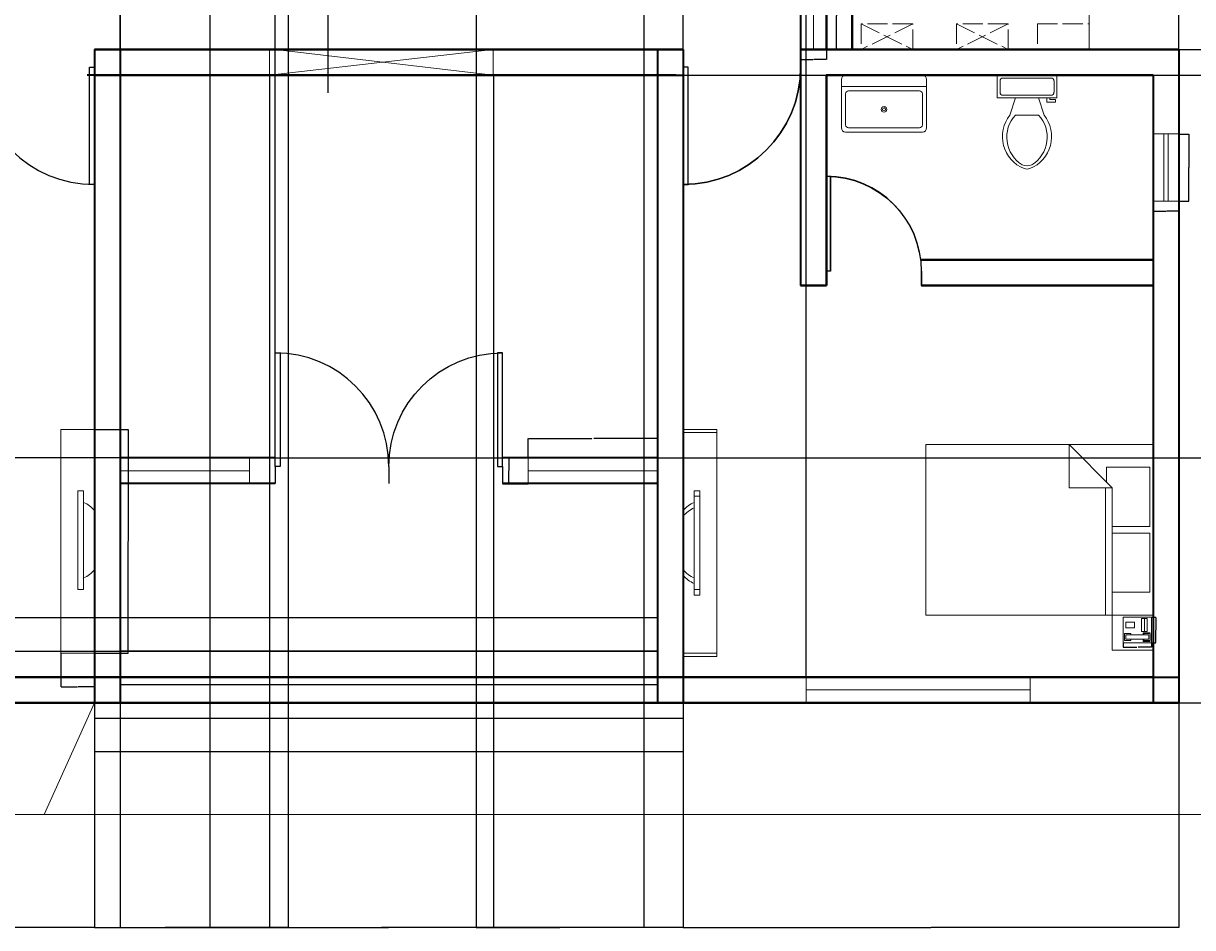
# Model space of a CAD drawing. Units: millimetres. Extents: x -8052 to 19968, y -37825 to -17505.
# Tile 3 of 10: x 84 to 10533, y -37825 to -29741. Entities that reach past the tile are written whole.
import ezdxf

# ---------------------------------------------------------------- set-up
doc = ezdxf.new("R2010")
doc.units = ezdxf.units.MM
doc.header["$MEASUREMENT"] = 0
doc.linetypes.add('ACAD_ISO02W100', pattern=[15, 12, -3])
for name, color, linetype, lineweight in [('A-ANNO-DIMS', 2, 'Continuous', 18), ('A-DOOR', 3, 'Continuous', 25), ('A-EQPM', 8, 'Continuous', 18), ('A-FLOR', 8, 'Continuous', 18), ('A-FLOR-FIXT', 9, 'Continuous', 18), ('A-FLOR-STRS', 7, 'Continuous', 25), ('A-FURN', 8, 'Continuous', 18), ('A-GLAZ', 4, 'Continuous', 18), ('A-ROOF-OVHD', 8, 'ACAD_ISO02W100', 18), ('A-WALL', 7, 'Continuous', 35)]:
    doc.layers.add(name, color=color, linetype=linetype, lineweight=lineweight)
doc.styles.get("Standard").update_dxf_attribs({"font": 'arial.ttf'})
doc.dimstyles.get("Standard").update_dxf_attribs({"dimtxt": 1.054, "dimasz": 1.055, "dimexe": 0.18, "dimexo": 0.0625, "dimgap": 0.09, "dimtad": 0, "dimtih": 1, "dimtoh": 1, "dimdec": 4, "dimzin": 0, "dimdsep": 46, "dimtxsty": 'Standard', "dimcen": 0.09, "dimadec": 0, "dimazin": 0, "dimtfac": 1, "dimtdec": 4, "dimtofl": 0, "dimtmove": 0, "dimatfit": 3, "dimfxl": 1, "dimtolj": 1, "dimtzin": 0, "dimarcsym": 0})

# ---------------------------------------------------------------- blocks, each defined once
blk = doc.blocks.new('*U18')
for p, q in [((0, 0), (0, -6)), ((-40, 0), (-40, -6))]:
    blk.add_line(p, q)
blk.add_lwpolyline([(0, 0), (0, 40), (-1.75, 40), (-1.75, 0)], close=True)
blk.add_arc((0, 0), 40, 90, 180)
blk = doc.blocks.new('*U10')
for p, q in [((0, 0), (0, -6)), ((40, 0), (40, -6))]:
    blk.add_line(p, q)
blk.add_lwpolyline([(0, 0), (0, 40), (1.75, 40), (1.75, 0)], close=True)
blk.add_arc((0, 0), 40, 0, 90)
blk = doc.blocks.new('*U19')
for p, q in [((0, 0), (0, -6)), ((40, 0), (40, -6))]:
    blk.add_line(p, q)
blk.add_lwpolyline([(0, 0), (0, 40), (1.75, 40), (1.75, 0)], close=True)
blk.add_arc((0, 0), 40, 0, 90)
blk = doc.blocks.new('*U17')
for p, q in [((0, 0), (0, 6)), ((40, 0), (40, 6))]:
    blk.add_line(p, q)
blk.add_lwpolyline([(0, 0), (0, -40), (1.75, -40), (1.75, 0)], close=True)
blk.add_arc((0, 0), 40, 270, 0)
blk = doc.blocks.new('Sink-single - 30 in top')
blk.add_line((-15, -3.999996), (15, -3.999996))
for points in [[(-13.5, 0), (13.5, 0)], [(-15, -18.499996), (-15, -1.5)], [(15, -1.5), (15, -18.499996)], [(-13.5, -17.499996), (-13.5, -6.499996)], [(-12.5, -5.499996), (12.5, -5.499996)], [(13.5, -6.499996), (13.5, -17.499996)], [(13.5, -19.999996), (-13.5, -19.999996)], [(12.5, -18.499996), (-12.5, -18.499996)]]:
    blk.add_lwpolyline(points)
for radius in [1, 0.5]:
    blk.add_circle((0, -11.999996), radius)
for centre, radius, start, end in [((-13.5, -1.5), 1.5, 90, 180), ((13.5, -1.5), 1.5, 0, 90), ((-12.5, -6.499996), 1, 90, 180), ((12.5, -6.499996), 1, 0, 90), ((-13.5, -18.499996), 1.5, 180, 270), ((-12.5, -17.499996), 1, 180, 270), ((12.5, -17.499996), 1, 270, 0), ((13.5, -18.499996), 1.5, 270, 0)]:
    blk.add_arc(centre, radius, start, end)
blk = doc.blocks.new('Toilet - top')
for p, q in [((9.5, -6), (9.5, -2)), ((-8, -8.5), (-8, -8)), ((-7, -8), (-7, -9.5)), ((-4, -8), (-6, -14)), ((4, -8), (6, -14)), ((-10, -8.5), (-8, -8.5)), ((-10, -9.5), (-10, -8.5)), ((-7, -9.5), (-10, -9.5)), ((4, -14), (-4, -14))]:
    blk.add_line(p, q)
blk.add_lwpolyline([(10.5, -8), (10.5, 0), (-10.5, 0), (-10.5, -8)], close=True)
for points in [[(-9.5, -2), (-9.5, -6)], [(8.5, -1), (-8.5, -1)], [(-8.5, -7), (8.5, -7)]]:
    blk.add_lwpolyline(points)
for centre, radius, start, end in [((-8.62, -1.88), 0.884, 81.8699, 188.1301), ((8.62, -1.88), 0.884, 351.8699, 98.1301), ((-8.62, -6.12), 0.884, 171.8699, 278.1301), ((8.62, -6.12), 0.884, 261.8699, 8.1301), ((3.52, -21.58), 12.17, 141.4691, 247.9714), ((4.2, -21.82), 11.33, 136.3677, 238.9468), ((-3.52, -21.58), 12.17, 292.0284, 38.5307), ((-4.2, -21.82), 11.33, 301.053, 43.6321), ((0, -27.88), 4, 245.7318, 294.2682), ((0, -29), 4, 254.8605, 285.1395)]:
    blk.add_arc(centre, radius, start, end)
blk = doc.blocks.new('Bed - Queen')
for p, q in [((0, -80.00003), (0, 0)), ((0, 0), (59.99999, 0)), ((59.99999, 0), (59.99999, -80.00003)), ((7.99999, -1.2), (28.79998, -1.2)), ((7.99999, -14.4), (7.99999, -1.2)), ((28.79998, -1.2), (28.79998, -14.4)), ((31.19999, -1.2), (51.99999, -1.2)), ((31.19999, -14.4), (31.19999, -1.2)), ((51.99999, -1.2), (51.99999, -16.4)), ((0, -14.4), (44.8, -14.4)), ((59.99999, -29.6), (44.8, -14.4)), ((44.8, -14.4), (44.8, -29.6)), ((51.99999, -16.4), (46.79936, -16.4)), ((44.8, -16.8), (0, -16.8)), ((44.8, -29.6), (59.99999, -29.6)), ((59.99999, -80.00003), (0, -80.00003))]:
    blk.add_line(p, q)
blk = doc.blocks.new('Phone - Desk')
for p, q in [((-4.5, -5), (-4.5, 5)), ((-4.5, 5), (4.5, 5)), ((-4, 4.5), (-4, 2)), ((-3.75, 4.5), (-3.75, 2.25)), ((-1.25, 4.5), (-3.75, 4.5)), ((-1.25, 2.25), (-1.25, 4.5)), ((-1, 2), (-1, 4.5)), ((4.5, 5), (4.5, -5)), ((-4, 2), (-3.25, 2)), ((-3.75, 2.25), (-3.25, 2.25)), ((-3.25, 4), (-3.25, -4)), ((-3.25, 4), (-1.75, 4)), ((-1.75, -4), (-1.75, 4)), ((-1.75, 2.25), (-1.25, 2.25)), ((-1.75, 2), (-1, 2)), ((4, 3.5), (-0.5, 3.5)), ((-0.5, 3.5), (-0.5, 1.5)), ((-0.5, 2.5), (4, 2.5)), ((-0.5, 1.5), (4, 1.5)), ((4, 1.5), (4, 3.5)), ((-3.75, -2.25), (-3.25, -2.25)), ((-3.75, -4.5), (-3.75, -2.25)), ((-3.25, -4), (-1.75, -4)), ((-1.75, -2.25), (-1.25, -2.25)), ((-1.25, -2.25), (-1.25, -4.5)), ((2.75, -1), (0.75, -1)), ((0.75, -1), (0.75, -4)), ((0.75, -4), (2.75, -4)), ((2.75, -4), (2.75, -1)), ((4.5, -5), (-4.5, -5)), ((-1.25, -4.5), (-3.75, -4.5))]:
    blk.add_line(p, q)
blk = doc.blocks.new('*U21')
for p, q in [((0, 0), (0, -6)), ((40, 0), (40, -6))]:
    blk.add_line(p, q)
blk.add_lwpolyline([(0, 0), (0, 40), (1.75, 40), (1.75, 0)], close=True)
blk.add_arc((0, 0), 40, 0, 90)
blk = doc.blocks.new('PERGOLA-CROSSED-MEMBER')
at = {"ltscale": 15}
for p, q in [((0, 230), (460, 0)), ((460, 230), (0, 0))]:
    blk.add_line(p, q, dxfattribs=at)
blk.add_lwpolyline([(0, 230), (460, 230), (460, 0), (0, 0)], close=True, dxfattribs=at)
blk = doc.blocks.new('TABLE-BEDSIDE')
for p, q in [((366, 315), (366, 0)), ((366, 0), (0, 0))]:
    blk.add_line(p, q)
blk = doc.blocks.new('MEDIA-CONSOLE-2000')
for points in [[(300, 2000), (0, 2000), (0, 0), (300, 0)], [(202, 1452), (152, 1452), (152, 569), (202, 569)], [(202, 569), (152, 569), (152, 1452), (202, 1452)]]:
    blk.add_lwpolyline(points, close=True)
for centre, start, end in [((115, 1133), 37.0745, 68.1008), ((115, 888), 291.8992, 322.9255)]:
    blk.add_arc(centre, 232, start, end)
blk = doc.blocks.new('WIN-2000')
for p, q in [((0, 0), (0, 230)), ((2000, 0), (2000, 230)), ((0, 115), (2000, 115))]:
    blk.add_line(p, q)
blk = doc.blocks.new('WIN-BATH-600')
for p, q in [((230, 600), (0, 600)), ((95, 600), (95, 0)), ((135, 600), (135, 0)), ((230, 0), (0, 0)), ((115, 0), (115, 0))]:
    blk.add_line(p, q)
blk = doc.blocks.new('WIN-SIDE-600')
for p, q in [((115, 0), (115, 600)), ((0, 0), (230, 0))]:
    blk.add_line(p, q)
blk = doc.blocks.new('WIN-ENTRY-1154')
for p, q in [((1154, 0), (1154, 230)), ((1154, 115), (0, 115))]:
    blk.add_line(p, q)
blk = doc.blocks.new('*D46')
at = {"layer": 'A-ANNO-DIMS', "color": 0, "lineweight": -2, "transparency": 16777216}
for p, q in [((720, -33371), (1020, -33371)), ((1020, -33372), (1020, -34371)), ((1020, -35370), (1020, -34372)), ((720, -35371), (1020, -35371))]:
    blk.add_line(p, q, dxfattribs=at)
at = {"layer": 'A-ANNO-DIMS', "color": 0, "lineweight": 100, "transparency": 16777216}
for points in [[(1020, -33372), (1020, -33372), (1020, -33371)], [(1020, -35370), (1020, -35370), (1020, -35371)]]:
    blk.add_solid(points, dxfattribs=at)
at = {"layer": 'Defpoints', "color": 0, "lineweight": 100, "transparency": 16777216}
for p in [(720, -33371), (1020, -33371), (720, -35371)]:
    blk.add_point(p, dxfattribs=at)
at = {"layer": 'A-ANNO-DIMS', "color": 0, "transparency": 16777216, "insert": (1020, -34371), "char_height": 1.05, "attachment_point": 5}
blk.add_mtext('\\A1;MEDIA CONSOLE 2000 TYP.', dxfattribs=at)
blk = doc.blocks.new('*D47')
at = {"layer": 'A-ANNO-DIMS', "color": 0, "lineweight": -2, "transparency": 16777216}
for p, q in [((420, -35371), (420, -35671)), ((720, -35371), (720, -35671)), ((421, -35671), (567, -35671)), ((719, -35671), (573, -35671))]:
    blk.add_line(p, q, dxfattribs=at)
at = {"layer": 'A-ANNO-DIMS', "color": 0, "lineweight": 100, "transparency": 16777216}
for points in [[(421, -35671), (421, -35671), (420, -35671)], [(719, -35671), (719, -35671), (720, -35671)]]:
    blk.add_solid(points, dxfattribs=at)
at = {"layer": 'Defpoints', "color": 0, "lineweight": 100, "transparency": 16777216}
for p in [(420, -35371), (720, -35371), (720, -35671)]:
    blk.add_point(p, dxfattribs=at)
at = {"layer": 'A-ANNO-DIMS', "color": 0, "transparency": 16777216, "insert": (570, -35671), "char_height": 1.05, "attachment_point": 5}
blk.add_mtext('\\A1;300 TYP.', dxfattribs=at)
blk = doc.blocks.new('*D48')
at = {"layer": 'A-ANNO-DIMS', "color": 0, "lineweight": -2, "transparency": 16777216}
for p, q in [((9912, -35278), (9912, -35317)), ((10166, -35278), (10166, -35317)), ((9913, -35317), (10033, -35317)), ((10165, -35317), (10045, -35317))]:
    blk.add_line(p, q, dxfattribs=at)
at = {"layer": 'A-ANNO-DIMS', "color": 0, "lineweight": 100, "transparency": 16777216}
for points in [[(9913, -35316), (9913, -35317), (9912, -35317)], [(10165, -35316), (10165, -35317), (10166, -35317)]]:
    blk.add_solid(points, dxfattribs=at)
at = {"layer": 'Defpoints', "color": 0, "lineweight": 100, "transparency": 16777216}
for p in [(9912, -35278), (10166, -35278), (10166, -35317)]:
    blk.add_point(p, dxfattribs=at)
at = {"layer": 'A-ANNO-DIMS', "color": 0, "transparency": 16777216, "insert": (10039, -35317), "char_height": 1.05, "attachment_point": 5}
blk.add_mtext('\\A1;PHONE 254 TYP.', dxfattribs=at)
blk = doc.blocks.new('*D49')
at = {"layer": 'A-ANNO-DIMS', "color": 0, "lineweight": -2, "transparency": 16777216}
for p, q in [((10166, -35050), (10204, -35050)), ((10204, -35051), (10204, -35164)), ((10204, -35277), (10204, -35165)), ((10166, -35278), (10204, -35278))]:
    blk.add_line(p, q, dxfattribs=at)
at = {"layer": 'A-ANNO-DIMS', "color": 0, "lineweight": 100, "transparency": 16777216}
for points in [[(10204, -35051), (10204, -35051), (10204, -35050)], [(10204, -35277), (10204, -35277), (10204, -35278)]]:
    blk.add_solid(points, dxfattribs=at)
at = {"layer": 'Defpoints', "color": 0, "lineweight": 100, "transparency": 16777216}
for p in [(10166, -35050), (10204, -35050), (10166, -35278)]:
    blk.add_point(p, dxfattribs=at)
at = {"layer": 'A-ANNO-DIMS', "color": 0, "transparency": 16777216, "insert": (10204, -35164), "char_height": 1.05, "attachment_point": 5}
blk.add_mtext('\\A1;229 TYP.', dxfattribs=at)
blk = doc.blocks.new('*D54')
at = {"layer": 'A-ANNO-DIMS', "color": 0, "lineweight": -2, "transparency": 16777216}
for p, q in [((7260, -29375), (7350, -29375)), ((7350, -29376), (7350, -29674)), ((7350, -29974), (7350, -29675)), ((7260, -29975), (7350, -29975))]:
    blk.add_line(p, q, dxfattribs=at)
at = {"layer": 'A-ANNO-DIMS', "color": 0, "lineweight": 100, "transparency": 16777216}
for points in [[(7350, -29376), (7350, -29376), (7350, -29375)], [(7350, -29974), (7350, -29974), (7350, -29975)]]:
    blk.add_solid(points, dxfattribs=at)
at = {"layer": 'Defpoints', "color": 0, "lineweight": 100, "transparency": 16777216}
for p in [(7260, -29375), (7260, -29975), (7350, -29975)]:
    blk.add_point(p, dxfattribs=at)
at = {"layer": 'A-ANNO-DIMS', "color": 0, "transparency": 16777216, "insert": (7350, -29675), "char_height": 1.05, "attachment_point": 5}
blk.add_mtext('\\A1;SIDE WINDOW 600 TYP.', dxfattribs=at)
blk = doc.blocks.new('*D55')
at = {"layer": 'A-ANNO-DIMS', "color": 0, "lineweight": -2, "transparency": 16777216}
for p, q in [((7030, -29975), (7030, -30065)), ((7260, -29975), (7260, -30065)), ((7031, -30065), (7142, -30065)), ((7259, -30065), (7148, -30065))]:
    blk.add_line(p, q, dxfattribs=at)
at = {"layer": 'A-ANNO-DIMS', "color": 0, "lineweight": 100, "transparency": 16777216}
for points in [[(7031, -30065), (7031, -30065), (7030, -30065)], [(7259, -30065), (7259, -30065), (7260, -30065)]]:
    blk.add_solid(points, dxfattribs=at)
at = {"layer": 'Defpoints', "color": 0, "lineweight": 100, "transparency": 16777216}
for p in [(7030, -29975), (7260, -29975), (7030, -30065)]:
    blk.add_point(p, dxfattribs=at)
at = {"layer": 'A-ANNO-DIMS', "color": 0, "transparency": 16777216, "insert": (7145, -30065), "char_height": 1.05, "attachment_point": 5}
blk.add_mtext('\\A1;230 TYP.', dxfattribs=at)
blk = doc.blocks.new('*D62')
at = {"layer": 'A-ANNO-DIMS', "color": 0, "lineweight": -2, "transparency": 16777216}
for p, q in [((10410, -30730), (10500, -30730)), ((10500, -30731), (10500, -31029)), ((10500, -31329), (10500, -31030)), ((10410, -31330), (10500, -31330))]:
    blk.add_line(p, q, dxfattribs=at)
at = {"layer": 'A-ANNO-DIMS', "color": 0, "lineweight": 100, "transparency": 16777216}
for points in [[(10500, -30731), (10500, -30731), (10500, -30730)], [(10500, -31329), (10500, -31329), (10500, -31330)]]:
    blk.add_solid(points, dxfattribs=at)
at = {"layer": 'Defpoints', "color": 0, "lineweight": 100, "transparency": 16777216}
for p in [(10410, -30730), (10500, -30730), (10410, -31330)]:
    blk.add_point(p, dxfattribs=at)
at = {"layer": 'A-ANNO-DIMS', "color": 0, "transparency": 16777216, "insert": (10500, -31030), "char_height": 1.05, "attachment_point": 5}
blk.add_mtext('\\A1;BATH WINDOW 600 TYP.', dxfattribs=at)
blk = doc.blocks.new('*D63')
at = {"layer": 'A-ANNO-DIMS', "color": 0, "lineweight": -2, "transparency": 16777216}
for p, q in [((10180, -31330), (10180, -31420)), ((10410, -31330), (10410, -31420)), ((10181, -31420), (10292, -31420)), ((10409, -31420), (10298, -31420))]:
    blk.add_line(p, q, dxfattribs=at)
at = {"layer": 'A-ANNO-DIMS', "color": 0, "lineweight": 100, "transparency": 16777216}
for points in [[(10181, -31420), (10181, -31420), (10180, -31420)], [(10409, -31420), (10409, -31420), (10410, -31420)]]:
    blk.add_solid(points, dxfattribs=at)
at = {"layer": 'Defpoints', "color": 0, "lineweight": 100, "transparency": 16777216}
for p in [(10180, -31330), (10410, -31330), (10410, -31420)]:
    blk.add_point(p, dxfattribs=at)
at = {"layer": 'A-ANNO-DIMS', "color": 0, "transparency": 16777216, "insert": (10295, -31420), "char_height": 1.05, "attachment_point": 5}
blk.add_mtext('\\A1;230 TYP.', dxfattribs=at)
blk = doc.blocks.new('*D66')
at = {"layer": 'A-ANNO-DIMS', "color": 0, "lineweight": -2, "transparency": 16777216}
for p, q in [((4596, -33625), (4596, -33452)), ((4597, -33452), (5163, -33452)), ((5749, -33452), (5183, -33452)), ((5750, -33625), (5750, -33452))]:
    blk.add_line(p, q, dxfattribs=at)
at = {"layer": 'A-ANNO-DIMS', "color": 0, "lineweight": 100, "transparency": 16777216}
for points in [[(4597, -33452), (4597, -33452), (4596, -33452)], [(5749, -33452), (5749, -33452), (5750, -33452)]]:
    blk.add_solid(points, dxfattribs=at)
at = {"layer": 'Defpoints', "color": 0, "lineweight": 100, "transparency": 16777216}
for p in [(4596, -33452), (4596, -33625), (5750, -33625)]:
    blk.add_point(p, dxfattribs=at)
at = {"layer": 'A-ANNO-DIMS', "color": 0, "transparency": 16777216, "insert": (5173, -33452), "char_height": 1.05, "attachment_point": 5}
blk.add_mtext('\\A1;ENTRY WINDOW 1154 TYP.', dxfattribs=at)
blk = doc.blocks.new('*D67')
at = {"layer": 'A-ANNO-DIMS', "color": 0, "lineweight": -2, "transparency": 16777216}
for p, q in [((4596, -33625), (4423, -33625)), ((4423, -33626), (4423, -33739)), ((4423, -33854), (4423, -33740)), ((4596, -33855), (4423, -33855))]:
    blk.add_line(p, q, dxfattribs=at)
at = {"layer": 'A-ANNO-DIMS', "color": 0, "lineweight": 100, "transparency": 16777216}
for points in [[(4423, -33626), (4423, -33626), (4423, -33625)], [(4423, -33854), (4423, -33854), (4423, -33855)]]:
    blk.add_solid(points, dxfattribs=at)
at = {"layer": 'Defpoints', "color": 0, "lineweight": 100, "transparency": 16777216}
for p in [(4596, -33625), (4423, -33855), (4596, -33855)]:
    blk.add_point(p, dxfattribs=at)
at = {"layer": 'A-ANNO-DIMS', "color": 0, "transparency": 16777216, "insert": (4423, -33740), "char_height": 1.05, "attachment_point": 5}
blk.add_mtext('\\A1;230 TYP.', dxfattribs=at)
blk = doc.blocks.new('*D95')
at = {"layer": 'A-ANNO-DIMS', "color": 0, "lineweight": -2, "transparency": 16777216}
for p, q in [((4130, -20745), (4130, -37825)), ((5630, -20745), (5630, -37825)), ((4131, -37824), (4878, -37824)), ((5629, -37824), (4882, -37824))]:
    blk.add_line(p, q, dxfattribs=at)
at = {"layer": 'A-ANNO-DIMS', "color": 0, "lineweight": 100, "transparency": 16777216}
for points in [[(4131, -37824), (4131, -37825), (4130, -37824)], [(5629, -37824), (5629, -37825), (5630, -37824)]]:
    blk.add_solid(points, dxfattribs=at)
at = {"layer": 'Defpoints', "color": 0, "lineweight": 100, "transparency": 16777216}
for p in [(4130, -20745), (5630, -20745), (5630, -37824)]:
    blk.add_point(p, dxfattribs=at)
at = {"layer": 'A-ANNO-DIMS', "color": 0, "transparency": 16777216, "insert": (4880, -37824), "char_height": 1.05, "attachment_point": 5}
blk.add_mtext('\\A1;1500', dxfattribs=at)
blk = doc.blocks.new('*D97')
at = {"layer": 'A-ANNO-DIMS', "color": 0, "lineweight": -2, "transparency": 16777216}
for p, q in [((12090, -25475), (14100, -25475)), ((14099, -25476), (14099, -27724)), ((14099, -29974), (14099, -27725)), ((10410, -29975), (14100, -29975))]:
    blk.add_line(p, q, dxfattribs=at)
at = {"layer": 'A-ANNO-DIMS', "color": 0, "lineweight": 100, "transparency": 16777216}
for points in [[(14099, -25476), (14100, -25476), (14099, -25475)], [(14099, -29974), (14100, -29974), (14099, -29975)]]:
    blk.add_solid(points, dxfattribs=at)
at = {"layer": 'Defpoints', "color": 0, "lineweight": 100, "transparency": 16777216}
for p in [(12090, -25475), (10410, -29975), (14099, -29975)]:
    blk.add_point(p, dxfattribs=at)
at = {"layer": 'A-ANNO-DIMS', "color": 0, "transparency": 16777216, "insert": (14099, -27725), "char_height": 1.05, "attachment_point": 5}
blk.add_mtext('\\A1;4500', dxfattribs=at)
blk = doc.blocks.new('*D98')
at = {"layer": 'A-ANNO-DIMS', "color": 0, "lineweight": -2, "transparency": 16777216}
for p, q in [((10410, -29975), (14100, -29975)), ((14099, -29976), (14099, -32894)), ((14099, -35814), (14099, -32895)), ((10410, -35815), (14100, -35815))]:
    blk.add_line(p, q, dxfattribs=at)
at = {"layer": 'A-ANNO-DIMS', "color": 0, "lineweight": 100, "transparency": 16777216}
for points in [[(14099, -29976), (14100, -29976), (14099, -29975)], [(14099, -35814), (14100, -35814), (14099, -35815)]]:
    blk.add_solid(points, dxfattribs=at)
at = {"layer": 'Defpoints', "color": 0, "lineweight": 100, "transparency": 16777216}
for p in [(10410, -29975), (10410, -35815), (14099, -35815)]:
    blk.add_point(p, dxfattribs=at)
at = {"layer": 'A-ANNO-DIMS', "color": 0, "transparency": 16777216, "insert": (14099, -32895), "char_height": 1.05, "attachment_point": 5}
blk.add_mtext('\\A1;5840', dxfattribs=at)
blk = doc.blocks.new('*D100')
at = {"layer": 'A-ANNO-DIMS', "color": 0, "lineweight": -2, "transparency": 16777216}
for p, q in [((-3710, -35815), (-3710, -37825)), ((720, -35815), (720, -37825)), ((-3709, -37824), (-1497, -37824)), ((719, -37824), (-1493, -37824))]:
    blk.add_line(p, q, dxfattribs=at)
at = {"layer": 'A-ANNO-DIMS', "color": 0, "lineweight": 100, "transparency": 16777216}
for points in [[(-3709, -37824), (-3709, -37825), (-3710, -37824)], [(719, -37824), (719, -37825), (720, -37824)]]:
    blk.add_solid(points, dxfattribs=at)
at = {"layer": 'Defpoints', "color": 0, "lineweight": 100, "transparency": 16777216}
for p in [(-3710, -35815), (720, -35815), (720, -37824)]:
    blk.add_point(p, dxfattribs=at)
at = {"layer": 'A-ANNO-DIMS', "color": 0, "transparency": 16777216, "insert": (-1495, -37824), "char_height": 1.05, "attachment_point": 5}
blk.add_mtext('\\A1;4430', dxfattribs=at)
blk = doc.blocks.new('*D101')
at = {"layer": 'A-ANNO-DIMS', "color": 0, "lineweight": -2, "transparency": 16777216}
for p, q in [((720, -35815), (720, -37825)), ((5980, -35815), (5980, -37825)), ((721, -37824), (3348, -37824)), ((5979, -37824), (3352, -37824))]:
    blk.add_line(p, q, dxfattribs=at)
at = {"layer": 'A-ANNO-DIMS', "color": 0, "lineweight": 100, "transparency": 16777216}
for points in [[(721, -37824), (721, -37825), (720, -37824)], [(5979, -37824), (5979, -37825), (5980, -37824)]]:
    blk.add_solid(points, dxfattribs=at)
at = {"layer": 'Defpoints', "color": 0, "lineweight": 100, "transparency": 16777216}
for p in [(720, -35815), (5980, -35815), (5980, -37824)]:
    blk.add_point(p, dxfattribs=at)
at = {"layer": 'A-ANNO-DIMS', "color": 0, "transparency": 16777216, "insert": (3350, -37824), "char_height": 1.05, "attachment_point": 5}
blk.add_mtext('\\A1;5260', dxfattribs=at)
blk = doc.blocks.new('*D102')
at = {"layer": 'A-ANNO-DIMS', "color": 0, "lineweight": -2, "transparency": 16777216}
for p, q in [((5980, -35815), (5980, -37825)), ((10410, -35815), (10410, -37825)), ((5981, -37824), (8193, -37824)), ((10409, -37824), (8197, -37824))]:
    blk.add_line(p, q, dxfattribs=at)
at = {"layer": 'A-ANNO-DIMS', "color": 0, "lineweight": 100, "transparency": 16777216}
for points in [[(5981, -37824), (5981, -37825), (5980, -37824)], [(10409, -37824), (10409, -37825), (10410, -37824)]]:
    blk.add_solid(points, dxfattribs=at)
at = {"layer": 'Defpoints', "color": 0, "lineweight": 100, "transparency": 16777216}
for p in [(5980, -35815), (10410, -35815), (10410, -37824)]:
    blk.add_point(p, dxfattribs=at)
at = {"layer": 'A-ANNO-DIMS', "color": 0, "transparency": 16777216, "insert": (8195, -37824), "char_height": 1.05, "attachment_point": 5}
blk.add_mtext('\\A1;4430', dxfattribs=at)
blk = doc.blocks.new('*D104')
at = {"layer": 'A-ANNO-DIMS', "color": 0, "lineweight": -2, "transparency": 16777216}
for p, q in [((5980, -35400), (5980, -17505)), ((5981, -17505), (6528, -17505)), ((7079, -17505), (6532, -17505)), ((7080, -35585), (7080, -17505))]:
    blk.add_line(p, q, dxfattribs=at)
at = {"layer": 'A-ANNO-DIMS', "color": 0, "lineweight": 100, "transparency": 16777216}
for points in [[(5981, -17505), (5981, -17506), (5980, -17505)], [(7079, -17505), (7079, -17506), (7080, -17505)]]:
    blk.add_solid(points, dxfattribs=at)
at = {"layer": 'Defpoints', "color": 0, "lineweight": 100, "transparency": 16777216}
for p in [(7080, -17505), (5980, -35400), (7080, -35585)]:
    blk.add_point(p, dxfattribs=at)
at = {"layer": 'A-ANNO-DIMS', "color": 0, "transparency": 16777216, "insert": (6530, -17505), "char_height": 1.05, "attachment_point": 5}
blk.add_mtext('\\A1;1100', dxfattribs=at)
blk = doc.blocks.new('*D108')
at = {"layer": 'A-ANNO-DIMS', "color": 0, "lineweight": -2, "transparency": 16777216}
for p, q in [((-330, -29975), (-330, -17505)), ((-329, -17505), (3348, -17505)), ((7029, -17505), (3352, -17505)), ((7030, -29975), (7030, -17505))]:
    blk.add_line(p, q, dxfattribs=at)
at = {"layer": 'A-ANNO-DIMS', "color": 0, "lineweight": 100, "transparency": 16777216}
for points in [[(-329, -17505), (-329, -17506), (-330, -17505)], [(7029, -17505), (7029, -17506), (7030, -17505)]]:
    blk.add_solid(points, dxfattribs=at)
at = {"layer": 'Defpoints', "color": 0, "lineweight": 100, "transparency": 16777216}
for p in [(7030, -17505), (-330, -29975), (7030, -29975)]:
    blk.add_point(p, dxfattribs=at)
at = {"layer": 'A-ANNO-DIMS', "color": 0, "transparency": 16777216, "insert": (3350, -17505), "char_height": 1.05, "attachment_point": 5}
blk.add_mtext('\\A1;7360', dxfattribs=at)
blk = doc.blocks.new('*D109')
at = {"layer": 'A-ANNO-DIMS', "color": 0, "lineweight": -2, "transparency": 16777216}
for p, q in [((720, -30205), (14100, -30205)), ((14099, -30206), (14099, -31914)), ((14099, -33624), (14099, -31915)), ((950, -33625), (14100, -33625))]:
    blk.add_line(p, q, dxfattribs=at)
at = {"layer": 'A-ANNO-DIMS', "color": 0, "lineweight": 100, "transparency": 16777216}
for points in [[(14099, -30206), (14100, -30206), (14099, -30205)], [(14099, -33624), (14100, -33624), (14099, -33625)]]:
    blk.add_solid(points, dxfattribs=at)
at = {"layer": 'Defpoints', "color": 0, "lineweight": 100, "transparency": 16777216}
for p in [(720, -30205), (950, -33625), (14099, -33625)]:
    blk.add_point(p, dxfattribs=at)
at = {"layer": 'A-ANNO-DIMS', "color": 0, "transparency": 16777216, "insert": (14099, -31915), "char_height": 1.05, "attachment_point": 5}
blk.add_mtext('\\A1;3420', dxfattribs=at)
blk = doc.blocks.new('*D113')
at = {"layer": 'A-ANNO-DIMS', "color": 0, "lineweight": -2, "transparency": 16777216}
for p, q in [((950, -25245), (950, -37825)), ((1750, -25245), (1750, -37825)), ((951, -37824), (1349, -37824)), ((1749, -37824), (1351, -37824))]:
    blk.add_line(p, q, dxfattribs=at)
at = {"layer": 'A-ANNO-DIMS', "color": 0, "lineweight": 100, "transparency": 16777216}
for points in [[(951, -37824), (951, -37825), (950, -37824)], [(1749, -37824), (1749, -37825), (1750, -37824)]]:
    blk.add_solid(points, dxfattribs=at)
at = {"layer": 'Defpoints', "color": 0, "lineweight": 100, "transparency": 16777216}
for p in [(950, -25245), (1750, -25245), (1750, -37824)]:
    blk.add_point(p, dxfattribs=at)
at = {"layer": 'A-ANNO-DIMS', "color": 0, "transparency": 16777216, "insert": (1350, -37824), "char_height": 1.05, "attachment_point": 5}
blk.add_mtext('\\A1;800', dxfattribs=at)
blk = doc.blocks.new('*D115')
at = {"layer": 'A-ANNO-DIMS', "color": 0, "lineweight": -2, "transparency": 16777216}
for p, q in [((950, -20745), (950, -37825)), ((2450, -20745), (2450, -37825)), ((951, -37824), (1698, -37824)), ((2449, -37824), (1702, -37824))]:
    blk.add_line(p, q, dxfattribs=at)
at = {"layer": 'A-ANNO-DIMS', "color": 0, "lineweight": 100, "transparency": 16777216}
for points in [[(951, -37824), (951, -37825), (950, -37824)], [(2449, -37824), (2449, -37825), (2450, -37824)]]:
    blk.add_solid(points, dxfattribs=at)
at = {"layer": 'Defpoints', "color": 0, "lineweight": 100, "transparency": 16777216}
for p in [(950, -20745), (2450, -20745), (2450, -37824)]:
    blk.add_point(p, dxfattribs=at)
at = {"layer": 'A-ANNO-DIMS', "color": 0, "transparency": 16777216, "insert": (1700, -37824), "char_height": 1.05, "attachment_point": 5}
blk.add_mtext('\\A1;1500', dxfattribs=at)
blk = doc.blocks.new('*D118')
at = {"layer": 'A-ANNO-DIMS', "color": 0, "lineweight": -2, "transparency": 16777216}
for p, q in [((950, -33625), (950, -17505)), ((951, -17505), (1640, -17505)), ((2333, -17505), (1644, -17505)), ((2334, -33625), (2334, -17505))]:
    blk.add_line(p, q, dxfattribs=at)
at = {"layer": 'A-ANNO-DIMS', "color": 0, "lineweight": 100, "transparency": 16777216}
for points in [[(951, -17505), (951, -17506), (950, -17505)], [(2333, -17505), (2333, -17506), (2334, -17505)]]:
    blk.add_solid(points, dxfattribs=at)
at = {"layer": 'Defpoints', "color": 0, "lineweight": 100, "transparency": 16777216}
for p in [(2334, -17505), (950, -33625), (2334, -33625)]:
    blk.add_point(p, dxfattribs=at)
at = {"layer": 'A-ANNO-DIMS', "color": 0, "transparency": 16777216, "insert": (1642, -17505), "char_height": 1.05, "attachment_point": 5}
blk.add_mtext('\\A1;1384', dxfattribs=at)
blk = doc.blocks.new('*D119')
at = {"layer": 'A-ANNO-DIMS', "color": 0, "lineweight": -2, "transparency": 16777216}
for p, q in [((5750, -35055), (-8050, -35055)), ((-8050, -35056), (-8050, -35204)), ((-8050, -35354), (-8050, -35205)), ((5750, -35355), (-8050, -35355))]:
    blk.add_line(p, q, dxfattribs=at)
at = {"layer": 'A-ANNO-DIMS', "color": 0, "lineweight": 100, "transparency": 16777216}
for points in [[(-8050, -35056), (-8049, -35056), (-8050, -35055)], [(-8050, -35354), (-8049, -35354), (-8050, -35355)]]:
    blk.add_solid(points, dxfattribs=at)
at = {"layer": 'Defpoints', "color": 0, "lineweight": 100, "transparency": 16777216}
for p in [(5750, -35055), (-8050, -35355), (5750, -35355)]:
    blk.add_point(p, dxfattribs=at)
at = {"layer": 'A-ANNO-DIMS', "color": 0, "transparency": 16777216, "insert": (-8050, -35205), "char_height": 1.05, "attachment_point": 5}
blk.add_mtext('\\A1;300', dxfattribs=at)
blk = doc.blocks.new('*D120')
at = {"layer": 'A-ANNO-DIMS', "color": 0, "lineweight": -2, "transparency": 16777216}
for p, q in [((950, -33625), (-8050, -33625)), ((-8050, -33626), (-8050, -34339)), ((-8050, -35054), (-8050, -34340)), ((950, -35055), (-8050, -35055))]:
    blk.add_line(p, q, dxfattribs=at)
at = {"layer": 'A-ANNO-DIMS', "color": 0, "lineweight": 100, "transparency": 16777216}
for points in [[(-8050, -33626), (-8049, -33626), (-8050, -33625)], [(-8050, -35054), (-8049, -35054), (-8050, -35055)]]:
    blk.add_solid(points, dxfattribs=at)
at = {"layer": 'Defpoints', "color": 0, "lineweight": 100, "transparency": 16777216}
for p in [(950, -33625), (-8050, -35055), (950, -35055)]:
    blk.add_point(p, dxfattribs=at)
at = {"layer": 'A-ANNO-DIMS', "color": 0, "transparency": 16777216, "insert": (-8050, -34340), "char_height": 1.05, "attachment_point": 5}
blk.add_mtext('\\A1;1430', dxfattribs=at)
blk = doc.blocks.new('*D121')
at = {"layer": 'A-ANNO-DIMS', "color": 0, "lineweight": -2, "transparency": 16777216}
for p, q in [((720, -30205), (720, -37825)), ((2284, -30205), (2284, -37825)), ((721, -37824), (1500, -37824)), ((2283, -37824), (1504, -37824))]:
    blk.add_line(p, q, dxfattribs=at)
at = {"layer": 'A-ANNO-DIMS', "color": 0, "lineweight": 100, "transparency": 16777216}
for points in [[(721, -37824), (721, -37825), (720, -37824)], [(2283, -37824), (2283, -37825), (2284, -37824)]]:
    blk.add_solid(points, dxfattribs=at)
at = {"layer": 'Defpoints', "color": 0, "lineweight": 100, "transparency": 16777216}
for p in [(720, -30205), (2284, -30205), (2284, -37824)]:
    blk.add_point(p, dxfattribs=at)
at = {"layer": 'A-ANNO-DIMS', "color": 0, "transparency": 16777216, "insert": (1502, -37824), "char_height": 1.05, "attachment_point": 5}
blk.add_mtext('\\A1;1563.7', dxfattribs=at)
blk = doc.blocks.new('*D122')
at = {"layer": 'A-ANNO-DIMS', "color": 0, "lineweight": -2, "transparency": 16777216}
for p, q in [((2284, -30205), (2284, -37825)), ((4284, -30205), (4284, -37825)), ((2285, -37824), (3282, -37824)), ((4283, -37824), (3285, -37824))]:
    blk.add_line(p, q, dxfattribs=at)
at = {"layer": 'A-ANNO-DIMS', "color": 0, "lineweight": 100, "transparency": 16777216}
for points in [[(2285, -37824), (2285, -37825), (2284, -37824)], [(4283, -37824), (4283, -37825), (4284, -37824)]]:
    blk.add_solid(points, dxfattribs=at)
at = {"layer": 'Defpoints', "color": 0, "lineweight": 100, "transparency": 16777216}
for p in [(2284, -30205), (4284, -30205), (4284, -37824)]:
    blk.add_point(p, dxfattribs=at)
at = {"layer": 'A-ANNO-DIMS', "color": 0, "transparency": 16777216, "insert": (3284, -37824), "char_height": 1.05, "attachment_point": 5}
blk.add_mtext('\\A1;2000', dxfattribs=at)
blk = doc.blocks.new('*D124')
at = {"layer": 'A-ANNO-DIMS', "color": 0, "lineweight": -2, "transparency": 16777216}
for p, q in [((7030, -29975), (7030, -17505)), ((7031, -17505), (8718, -17505)), ((10409, -17505), (8722, -17505)), ((10410, -29975), (10410, -17505))]:
    blk.add_line(p, q, dxfattribs=at)
at = {"layer": 'A-ANNO-DIMS', "color": 0, "lineweight": 100, "transparency": 16777216}
for points in [[(7031, -17505), (7031, -17506), (7030, -17505)], [(10409, -17505), (10409, -17506), (10410, -17505)]]:
    blk.add_solid(points, dxfattribs=at)
at = {"layer": 'Defpoints', "color": 0, "lineweight": 100, "transparency": 16777216}
for p in [(10410, -17505), (7030, -29975), (10410, -29975)]:
    blk.add_point(p, dxfattribs=at)
at = {"layer": 'A-ANNO-DIMS', "color": 0, "transparency": 16777216, "insert": (8720, -17505), "char_height": 1.05, "attachment_point": 5}
blk.add_mtext('\\A1;3380', dxfattribs=at)
blk = doc.blocks.new('*D136')
at = {"layer": 'A-ANNO-DIMS', "color": 0, "lineweight": -2, "transparency": 16777216}
for p, q in [((2808, -28110), (2808, -28110)), ((2808, -28110), (2808, -28110)), ((2808, -30361), (2808, -29518)), ((2807, -30361), (2808, -30361))]:
    blk.add_line(p, q, dxfattribs=at)
at = {"layer": 'A-ANNO-DIMS', "color": 0, "lineweight": 100, "transparency": 16777216}
blk.add_solid([(2808, -29518), (2808, -29518), (2808, -29517)], dxfattribs=at)
at = {"layer": 'Defpoints', "color": 0, "lineweight": 100, "transparency": 16777216}
for p in [(2808, -28110), (2808, -29517)]:
    blk.add_point(p, dxfattribs=at)
at = {"layer": 'A-ANNO-DIMS', "color": 0, "transparency": 16777216, "insert": (2803, -30361), "char_height": 1.05, "attachment_point": 5}
blk.add_mtext('\\A1;2X R1406.8', dxfattribs=at)

msp = doc.modelspace()

# ---------------------------------------------------------------- linework, layer by layer
at = {"layer": 'A-FLOR'}
for p, q in [((9607.479, -25474.843), (9607.479, -29974.843)), ((9607.479, -25474.843), (9607.479, -29974.843)), ((269.979, -36814.843), (719.979, -35814.843)), ((-4710.021, -36814.843), (11409.979, -36814.843))]:
    msp.add_line(p, q, dxfattribs=at)
at = {"layer": 'A-FLOR-STRS'}
for p, q in [((5749.979, -35054.843), (949.979, -35054.843)), ((5749.979, -35354.843), (949.979, -35354.843)), ((5749.979, -35654.843), (949.979, -35654.843)), ((719.979, -35814.843), (719.979, -35814.843)), ((719.979, -35814.843), (719.979, -36814.843)), ((5979.979, -35814.843), (5979.979, -36814.843)), ((5979.979, -35954.843), (719.979, -35954.843)), ((5979.979, -36254.843), (719.979, -36254.843))]:
    msp.add_line(p, q, dxfattribs=at)
at = {"layer": 'A-GLAZ'}
for p, q in [((2283.667, -30204.843), (2283.667, -29974.843)), ((2283.667, -30204.843), (4283.667, -29974.843)), ((2284.577, -29967.064), (4283.667, -30204.843)), ((2349.979, -29974.843), (2349.979, -29974.843)), ((4283.667, -30204.843), (4283.667, -29974.843))]:
    msp.add_line(p, q, dxfattribs=at)
at = {"layer": 'A-ROOF-OVHD', "ltscale": 15}
for q in [(9146.002, -29974.843), (9607.479, -29744.843)]:
    msp.add_line((9146.002, -29744.843), q, dxfattribs=at)
at = {"layer": 'A-WALL'}
for p, q in [((7259.979, -29974.843), (7259.979, -25474.843)), ((7259.979, -25474.843), (7259.979, -29974.843)), ((7489.979, -29974.843), (7489.979, -25474.843)), ((7489.979, -25474.843), (7489.979, -29974.843)), ((7029.979, -28740.843), (7029.979, -29974.843)), ((719.979, -29974.843), (719.979, -35814.843)), ((719.979, -29974.843), (5979.979, -29974.843)), ((3603.065, -29974.843), (719.979, -29974.843)), ((949.979, -29974.843), (949.979, -35814.843)), ((5979.979, -29974.843), (3603.065, -29974.843)), ((5749.979, -29974.843), (5749.979, -35814.843)), ((5749.979, -29974.843), (5749.979, -35814.843)), ((5979.979, -29974.843), (5979.979, -35814.843)), ((5979.979, -29974.843), (5979.979, -35814.843)), ((7029.979, -29974.843), (7029.979, -32084.843)), ((7029.979, -29974.843), (10409.979, -29974.843)), ((10409.979, -29974.843), (7029.979, -29974.843)), ((10409.979, -29974.843), (10409.979, -35814.843)), ((10409.979, -29974.843), (10409.979, -35814.843)), ((4283.667, -30204.843), (653.667, -30204.843)), ((719.979, -30204.843), (2283.667, -30204.843)), ((2283.667, -30204.843), (5979.979, -30204.843)), ((5913.667, -30204.843), (4283.667, -30204.843)), ((7027.473, -30204.843), (7029.979, -30204.843)), ((7027.473, -30204.843), (7027.473, -32084.843)), ((10179.979, -30204.843), (7257.473, -30204.843)), ((7257.473, -30204.843), (7257.473, -32084.843)), ((7259.979, -30204.843), (7259.979, -32084.843)), ((7259.979, -30204.843), (10179.979, -30204.843)), ((10179.979, -30204.843), (10179.979, -35814.843)), ((10179.979, -30204.843), (10179.979, -35584.843)), ((10179.979, -31854.843), (8101.271, -31854.843)), ((8109.979, -31854.843), (10179.979, -31854.843)), ((7257.473, -32084.843), (7027.473, -32084.843)), ((7029.979, -32084.843), (7259.979, -32084.843)), ((10179.979, -32084.843), (8107.473, -32084.843)), ((8109.979, -32084.843), (10179.979, -32084.843)), ((2333.979, -33624.843), (949.979, -33624.843)), ((3352.947, -33624.843), (3347.012, -33624.843)), ((5749.979, -33624.843), (4365.979, -33624.843)), ((2333.979, -33854.843), (949.979, -33854.843)), ((2333.979, -33854.843), (2103.979, -33854.843)), ((5749.979, -33854.843), (4365.979, -33854.843)), ((4365.979, -33854.843), (4595.979, -33854.843)), ((10179.979, -35584.843), (-3710.021, -35584.843)), ((-3480.021, -35584.843), (10409.979, -35584.843)), ((-3710.021, -35814.843), (10409.979, -35814.843)), ((10409.979, -35814.843), (-3710.021, -35814.843))]:
    msp.add_line(p, q, dxfattribs=at)

# ---------------------------------------------------------------- block references
at = {"layer": 'A-DOOR', "rotation": 180}
for name, p, xscale, yscale, zscale in [('*U10', (719.979, -30132.343), 26.25, 26.25, 26.25), ('*U18', (5979.979, -30132.343), 26.25000000000002, 26.25000000000002, 26.25000000000002), ('*U10', (5979.979, -30132.343), -26.25, 26.25, 26.25), ('*U18', (5979.979, -30132.343), 26.25000000000002, 26.25000000000002, 26.25000000000002), ('*U10', (5979.979, -30132.343), -26.25, 26.25, 26.25), ('*U17', (7257.473, -31957.343), -21.25, 21.25, 21.25)]:
    msp.add_blockref(name, p, dxfattribs=dict(at, xscale=xscale, yscale=yscale, zscale=zscale))
at = {"layer": 'A-DOOR'}
for name, p, xscale, yscale, zscale in [('*U19', (7259.979, -31957.343), 21.25, 21.25, 21.25), ('*U21', (2333.979, -33702.443), 25.39999999999996, 25.39999999999996, 25.39999999999996)]:
    msp.add_blockref(name, p, dxfattribs=dict(at, xscale=xscale, yscale=yscale, zscale=zscale))
at = {"layer": 'A-DOOR', "extrusion": (0, 0, -1), "xscale": 25.39999999999994, "yscale": 25.39999999999994, "zscale": -25.4}
msp.add_blockref('*U21', (-4365.979, -33702.443), dxfattribs=at)
at = {"layer": 'A-EQPM'}
msp.add_blockref('MEDIA-CONSOLE-2000', (419.979, -35371.308), dxfattribs=at)
at = {"layer": 'A-EQPM', "extrusion": (0, 0, -1), "zscale": -1}
msp.add_blockref('MEDIA-CONSOLE-2000', (-6279.98, -35371.308), dxfattribs=at)
at = {"layer": 'A-EQPM', "rotation": 180}
msp.add_blockref('MEDIA-CONSOLE-2000', (6279.98, -33400.039), dxfattribs=at)
at = {"layer": 'A-EQPM', "xscale": -25.4, "yscale": 25.4, "zscale": 25.4, "rotation": 270}
msp.add_blockref('Phone - Desk', (10038.719, -35164.132), dxfattribs=at)
at = {"layer": 'A-FLOR-FIXT', "xscale": -25.4, "yscale": 25.4, "zscale": 25.4}
for name, p in [('Sink-single - 30 in top', (7774.818, -30204.843)), ('Toilet - top', (9052.68, -30204.843))]:
    msp.add_blockref(name, p, dxfattribs=at)
at = {"layer": 'A-FURN', "xscale": -25.4, "yscale": 25.4, "zscale": 25.4, "rotation": 270}
msp.add_blockref('Bed - Queen', (10179.979, -35030.504), dxfattribs=at)
at = {"layer": 'A-FURN', "extrusion": (0, 0, -1), "zscale": -1}
msp.add_blockref('TABLE-BEDSIDE', (-10179.98, -35345.763), dxfattribs=at)
at = {"layer": 'A-GLAZ', "rotation": 180}
for name, p in [('WIN-SIDE-600', (7259.98, -29374.843)), ('WIN-ENTRY-1154', (5749.98, -33624.843))]:
    msp.add_blockref(name, p, dxfattribs=at)
at = {"layer": 'A-GLAZ'}
for name, p in [('WIN-BATH-600', (10179.979, -31329.843)), ('WIN-ENTRY-1154', (949.979, -33854.843)), ('WIN-2000', (7079.979, -35814.843))]:
    msp.add_blockref(name, p, dxfattribs=at)
at = {"layer": 'A-ROOF-OVHD', "extrusion": (0, 0, -1), "zscale": -1}
for p in [(-8031.275, -29974.843), (-8883.837, -29974.843)]:
    msp.add_blockref('PERGOLA-CROSSED-MEMBER', p, dxfattribs=at)

# ---------------------------------------------------------------- dimensions: what is measured, and where the dimension line sits
at = {"layer": 'A-ANNO-DIMS'}
for base, p1, p2, override, picture, middle in [((7029.979, -17505.343), (-330.021, -29974.843), (7029.979, -29974.843), {"dimdec": 0, "dimlfac": 1, "dimrnd": 0, "dimzin": 0, "dimdsep": 46, "dimlunit": 2}, '*D108', (3349.979, -17505.343)), ((2333.979, -17505.343), (949.979, -33624.843), (2333.979, -33624.843), {"dimdec": 0, "dimlfac": 1, "dimrnd": 0, "dimzin": 0, "dimdsep": 46, "dimlunit": 2}, '*D118', (1641.979, -17505.343)), ((7079.979, -17505.343), (5979.979, -35400.039), (7079.979, -35584.843), {"dimdec": 0, "dimlfac": 1, "dimrnd": 0, "dimzin": 0, "dimdsep": 46, "dimlunit": 2}, '*D104', (6529.979, -17505.343)), ((10409.979, -17505.343), (7029.979, -29974.843), (10409.979, -29974.843), {"dimdec": 0, "dimlfac": 1, "dimrnd": 0, "dimzin": 0, "dimdsep": 46, "dimlunit": 2}, '*D124', (8719.979, -17505.343)), ((2449.979, -37824.343), (949.979, -20744.843), (2449.979, -20744.843), {"dimdec": 0, "dimlfac": 1, "dimrnd": 0, "dimzin": 0, "dimdsep": 46, "dimlunit": 2}, '*D115', (1699.979, -37824.343)), ((5629.979, -37824.343), (4129.979, -20744.843), (5629.979, -20744.843), {"dimdec": 0, "dimlfac": 1, "dimrnd": 0, "dimzin": 0, "dimdsep": 46, "dimlunit": 2}, '*D95', (4879.979, -37824.343)), ((1749.979, -37824.343), (949.979, -25244.843), (1749.979, -25244.843), {"dimdec": 0, "dimlfac": 1, "dimrnd": 0, "dimzin": 0, "dimdsep": 46, "dimlunit": 2}, '*D113', (1349.979, -37824.343)), ((2283.667, -37824.343), (719.979, -30204.843), (2283.667, -30204.843), {"dimdec": 1, "dimlfac": 1, "dimrnd": 0, "dimzin": 0, "dimdsep": 46, "dimlunit": 2}, '*D121', (1501.823, -37824.343)), ((4283.667, -37824.343), (2283.667, -30204.843), (4283.667, -30204.843), {"dimdec": 0, "dimlfac": 1, "dimrnd": 0, "dimzin": 0, "dimdsep": 46, "dimlunit": 2}, '*D122', (3283.667, -37824.343)), ((719.979, -37824.343), (-3710.021, -35814.843), (719.979, -35814.843), {"dimdec": 0, "dimlfac": 1, "dimrnd": 0, "dimzin": 0, "dimdsep": 46, "dimlunit": 2}, '*D100', (-1495.021, -37824.343)), ((5979.979, -37824.343), (719.979, -35814.843), (5979.979, -35814.843), {"dimdec": 0, "dimlfac": 1, "dimrnd": 0, "dimzin": 0, "dimdsep": 46, "dimlunit": 2}, '*D101', (3349.979, -37824.343)), ((10409.979, -37824.343), (5979.979, -35814.843), (10409.979, -35814.843), {"dimdec": 0, "dimlfac": 1, "dimrnd": 0, "dimzin": 0, "dimdsep": 46, "dimlunit": 2}, '*D102', (8194.979, -37824.343))]:
    dim = msp.add_linear_dim(base=base, p1=p1, p2=p2, dimstyle='Standard', override=override, dxfattribs=at)
    dim.commit()
    dim.dimension.update_dxf_attribs({"geometry": picture, "text_midpoint": middle})
for base, p1, p2, picture, middle in [((14099.479, -29974.843), (12089.979, -25474.843), (10409.979, -29974.843), '*D97', (14099.479, -27724.843)), ((14099.479, -35814.843), (10409.979, -29974.843), (10409.979, -35814.843), '*D98', (14099.479, -32894.843)), ((14099.479, -33624.843), (719.979, -30204.843), (949.979, -33624.843), '*D109', (14099.479, -31914.843)), ((-8049.521, -35054.843), (949.979, -33624.843), (949.979, -35054.843), '*D120', (-8049.521, -34339.843)), ((-8049.521, -35354.843), (5749.979, -35054.843), (5749.979, -35354.843), '*D119', (-8049.521, -35204.843))]:
    dim = msp.add_linear_dim(base=base, p1=p1, p2=p2, angle=90, dimstyle='Standard', override={"dimdec": 0, "dimlfac": 1, "dimrnd": 0, "dimzin": 0, "dimdsep": 46, "dimlunit": 2}, dxfattribs=at)
    dim.commit()
    dim.dimension.update_dxf_attribs({"geometry": picture, "text_midpoint": middle})
dim = msp.add_radius_dim(center=(2808.199, -28110.126), mpoint=(2808.199, -29516.891), text='2X <>', dimstyle='Standard', override={"dimdec": 1, "dimlfac": 1, "dimrnd": 0, "dimzin": 0, "dimdsep": 46, "dimlunit": 2}, dxfattribs=at)
dim.commit()
dim.dimension.update_dxf_attribs({"geometry": '*D136', "text_midpoint": (2803.219, -30360.95), "dimtype": 164})
for base, p1, p2, angle, text, picture, middle in [((7349.979, -29974.843), (7259.979, -29374.843), (7259.979, -29974.843), 270, 'SIDE WINDOW <> TYP.', '*D54', (7349.979, -29674.843)), ((7029.979, -30064.843), (7259.979, -29974.843), (7029.979, -29974.843), 180, '<> TYP.', '*D55', (7144.979, -30064.843)), ((10499.979, -30729.843), (10409.979, -31329.843), (10409.979, -30729.843), 90, 'BATH WINDOW <> TYP.', '*D62', (10499.979, -31029.843)), ((1019.979, -33371.308), (719.979, -35371.308), (719.979, -33371.308), 90, 'MEDIA CONSOLE <> TYP.', '*D46', (1019.979, -34371.308)), ((4595.979, -33451.743), (5749.979, -33624.843), (4595.979, -33624.843), 180, 'ENTRY WINDOW <> TYP.', '*D66', (5172.979, -33451.743)), ((4422.879, -33854.843), (4595.979, -33624.843), (4595.979, -33854.843), 270, '<> TYP.', '*D67', (4422.879, -33739.843)), ((10203.819, -35049.832), (10165.719, -35278.432), (10165.719, -35049.832), 90, '<> TYP.', '*D49', (10203.819, -35164.132))]:
    dim = msp.add_linear_dim(base=base, p1=p1, p2=p2, angle=angle, text=text, dimstyle='Standard', override={"dimdec": 0, "dimlfac": 1, "dimrnd": 0, "dimzin": 0, "dimdsep": 46, "dimlunit": 2}, dxfattribs=at)
    dim.commit()
    dim.dimension.update_dxf_attribs({"geometry": picture, "text_midpoint": middle})
for base, p1, p2, text, picture, middle in [((10409.979, -31419.843), (10179.979, -31329.843), (10409.979, -31329.843), '<> TYP.', '*D63', (10294.979, -31419.843)), ((10165.719, -35316.532), (9911.719, -35278.432), (10165.719, -35278.432), 'PHONE <> TYP.', '*D48', (10038.719, -35316.532)), ((719.979, -35671.308), (419.979, -35371.308), (719.979, -35371.308), '<> TYP.', '*D47', (569.979, -35671.308))]:
    dim = msp.add_linear_dim(base=base, p1=p1, p2=p2, text=text, dimstyle='Standard', override={"dimdec": 0, "dimlfac": 1, "dimrnd": 0, "dimzin": 0, "dimdsep": 46, "dimlunit": 2}, dxfattribs=at)
    dim.commit()
    dim.dimension.update_dxf_attribs({"geometry": picture, "text_midpoint": middle})

doc.saveas('drawing.dxf')
